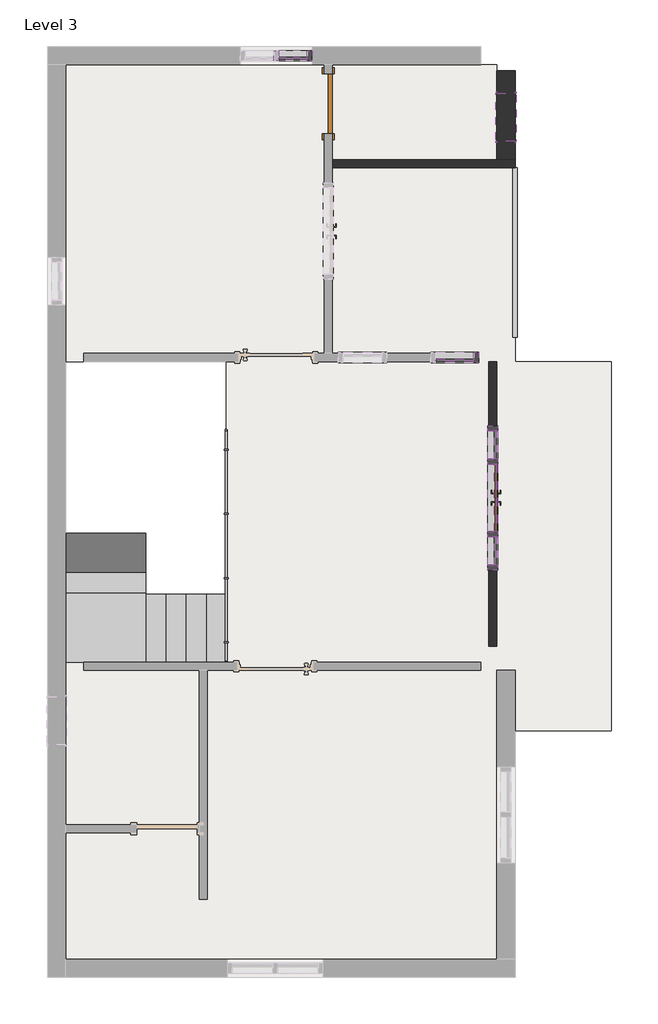
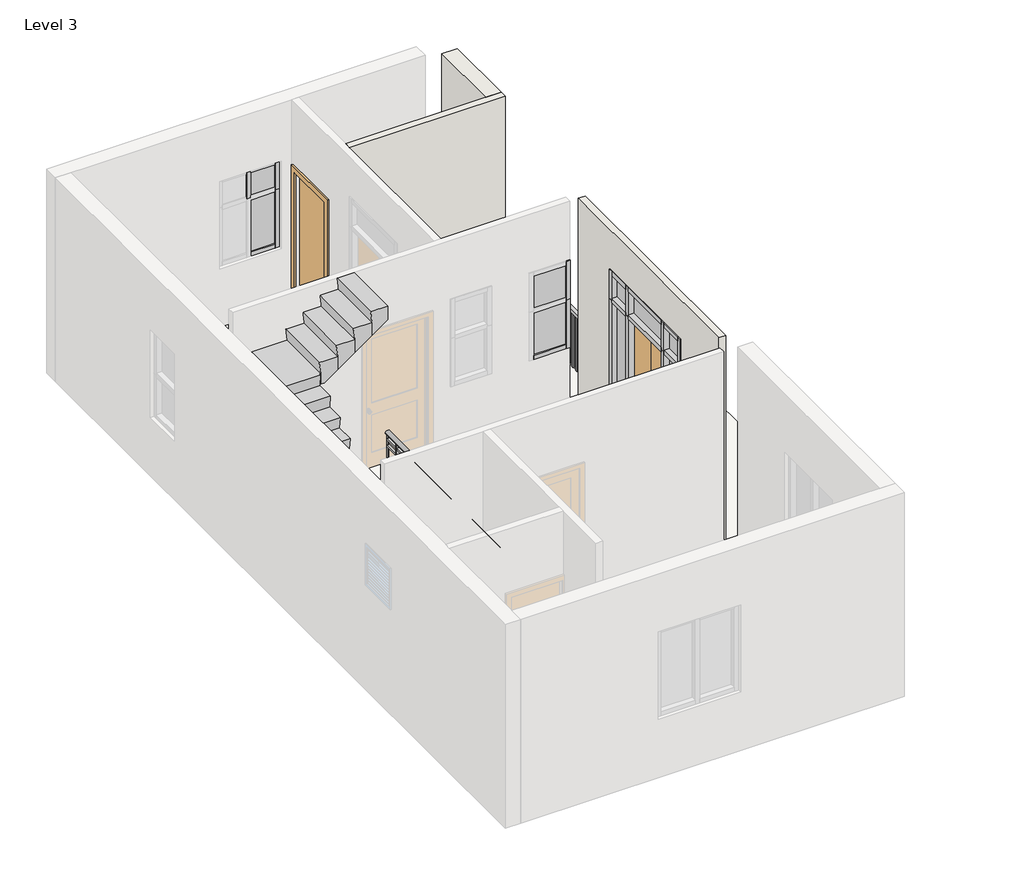
# One storey, part 2 of 2: 24 members, 9 plates, 3 walls, 2 doors, 2 railings, 1 slab, 1 stair flight, 1 window.
"""IFC4 building model written with IfcOpenShell, lengths in millimetres."""

from ifc_helpers import new_model, si_unit, point, frame, origin, place, context, project, spatial, polyline, ellipse_curve, trimmed, outline, extrude, faceted_brep, transform, mapped, element, save
from ifc_brep_helpers import plane_surface, extruded_surface, advanced_brep
from components import door_curtain_wall_double_glass_door_curtain_wall_double_88735db7, door_aa9e95e7, member_ffd4c858, member_15823cb3, member_843225dc, member_7cbddb58, member_af2f84b9, member_7db1855a, member_d2e7e466, member_3374d9b6, member_86d06fe4, member_47bfaf8a, member_aa870034, member_73c23c35, system_panel_glazed_a2bc0953, system_panel_glazed_235599b7, system_panel_glazed_0c1cb5df, system_panel_glazed_afbb4b88, system_panel_glazed_c43f0a09, system_panel_glazed_cc98a0ec, window_f2d8fef0

model = new_model("IFC4")

# Units and contexts
model_context = context("Model", 3, world=origin())
ifc_project = project(units=[si_unit("LENGTHUNIT", "METRE", prefix="MILLI")], contexts=[model_context])

# Site, building, storey
site = spatial("IfcSite", under=ifc_project)
building = spatial("IfcBuilding", under=site)
storey = spatial("IfcBuildingStorey", under=building, Name="Level 3", Elevation=3810.0)

# Doors
placement = place(None, origin())
door_curtain_wall_double_glass_door_curtain_wall_double_shape = door_curtain_wall_double_glass_door_curtain_wall_double_88735db7(model_context)
element("IfcDoor", 1, ObjectType="Door-Curtain-Wall-Double-Glass : Door-Curtain-Wall-Double-Glass", at=placement, inside=storey, context=model_context, shape_type="MappedRepresentation", body=[
    mapped(door_curtain_wall_double_glass_door_curtain_wall_double_shape, transform((576.4834347, 1882.9857557, 3873.5), x_axis=(0.0, -1.0, 0.0), y_axis=(1.0, 0.0, 0.0), z_axis=(0.0, 0.0, 1.0))),
])
door_shape = door_aa9e95e7(model_context)
element("IfcDoor", 2, ObjectType="Single-Flush : 2'6\" x7'", at=placement, inside=storey, context=model_context, shape_type="MappedRepresentation", body=[
    mapped(door_shape, transform((-1506.3165653, 6874.0857557, 3810.0), x_axis=(0.0, 1.0, 0.0), y_axis=(-1.0, 0.0, 0.0), z_axis=(0.0, 0.0, 1.0))),
])

# Members
member_shape = member_ffd4c858(model_context)
element("IfcMember", 3, ObjectType="Rectangular Mullion : 2.5\" x 5\" rectangular", at=placement, inside=storey, context=model_context, shape_type="MappedRepresentation", body=[
    mapped(member_shape, transform((576.4834347, 1425.7857557, 5943.6), x_axis=(0.0, -1.0, 0.0), y_axis=(-1.0, 0.0, 0.0), z_axis=(0.0, 0.0, -1.0))),
])
element("IfcMember", 4, ObjectType="Rectangular Mullion : 2.5\" x 5\" rectangular", at=placement, inside=storey, context=model_context, shape_type="MappedRepresentation", body=[
    mapped(member_shape, transform((576.4834347, 2340.1857557, 5943.6), x_axis=(0.0, -1.0, 0.0), y_axis=(-1.0, 0.0, 0.0), z_axis=(0.0, 0.0, -1.0))),
])
element("IfcMember", 5, ObjectType="Rectangular Mullion : 2.5\" x 5\" rectangular", at=placement, inside=storey, context=model_context, shape_type="MappedRepresentation", body=[
    mapped(member_shape, transform((-2166.7165653, 7483.6857557, 5638.8), x_axis=(-1.0, 0.0, 0.0), y_axis=(0.0, 1.0, 0.0), z_axis=(0.0, 0.0, -1.0))),
])
member_2_shape = member_15823cb3(model_context)
element("IfcMember", 6, ObjectType="Rectangular Mullion : 2.5\" x 5\" rectangular", at=placement, inside=storey, context=model_context, shape_type="MappedRepresentation", body=[
    mapped(member_2_shape, transform((576.4834347, 2797.3857557, 6400.8), x_axis=(0.0, 1.0, 0.0), y_axis=(-1.0, 0.0, 0.0), z_axis=(0.0, 0.0, 1.0))),
])
element("IfcMember", 7, ObjectType="Rectangular Mullion : 2.5\" x 5\" rectangular", at=placement, inside=storey, context=model_context, shape_type="MappedRepresentation", body=[
    mapped(member_2_shape, transform((-1709.5165653, 7483.6857557, 6096.0), x_axis=(1.0, 0.0, 0.0), y_axis=(0.0, 1.0, 0.0), z_axis=(0.0, 0.0, 1.0))),
])
element("IfcMember", 8, ObjectType="Rectangular Mullion : 2.5\" x 5\" rectangular", at=placement, inside=storey, context=model_context, shape_type="MappedRepresentation", body=[
    mapped(member_2_shape, transform((576.4834347, 968.5857557, 5943.6), x_axis=(0.0, -1.0, 0.0), y_axis=(-1.0, 0.0, 0.0), z_axis=(0.0, 0.0, -1.0))),
])
member_3_shape = member_843225dc(model_context)
element("IfcMember", 9, ObjectType="Rectangular Mullion : 2.5\" x 5\" rectangular", at=placement, inside=storey, context=model_context, shape_type="MappedRepresentation", body=[
    mapped(member_3_shape, transform((576.4834347, 1032.0857557, 6400.8), x_axis=(0.0, 0.0, 1.0), y_axis=(-1.0, 0.0, 0.0), z_axis=(0.0, -1.0, 0.0))),
])
element("IfcMember", 10, ObjectType="Rectangular Mullion : 2.5\" x 5\" rectangular", at=placement, inside=storey, context=model_context, shape_type="MappedRepresentation", body=[
    mapped(member_3_shape, transform((576.4834347, 2371.9357557, 6400.8), x_axis=(0.0, 0.0, 1.0), y_axis=(-1.0, 0.0, 0.0), z_axis=(0.0, -1.0, 0.0))),
])
element("IfcMember", 11, ObjectType="Rectangular Mullion : 2.5\" x 5\" rectangular", at=placement, inside=storey, context=model_context, shape_type="MappedRepresentation", body=[
    mapped(member_3_shape, transform((576.4834347, 2733.8857557, 3810.0), x_axis=(0.0, 0.0, -1.0), y_axis=(-1.0, 0.0, 0.0), z_axis=(0.0, 1.0, 0.0))),
])
element("IfcMember", 12, ObjectType="Rectangular Mullion : 2.5\" x 5\" rectangular", at=placement, inside=storey, context=model_context, shape_type="MappedRepresentation", body=[
    mapped(member_3_shape, transform((576.4834347, 1394.0357557, 3810.0), x_axis=(0.0, 0.0, -1.0), y_axis=(-1.0, 0.0, 0.0), z_axis=(0.0, 1.0, 0.0))),
])
element("IfcMember", 13, ObjectType="Rectangular Mullion : 2.5\" x 5\" rectangular", at=placement, inside=storey, context=model_context, shape_type="MappedRepresentation", body=[
    mapped(member_3_shape, transform((-1773.0165653, 7483.6857557, 4724.4), x_axis=(0.0, 0.0, -1.0), y_axis=(0.0, 1.0, 0.0), z_axis=(1.0, 0.0, 0.0))),
])
member_4_shape = member_7cbddb58(model_context)
element("IfcMember", 14, ObjectType="Rectangular Mullion : 2.5\" x 5\" rectangular", at=placement, inside=storey, context=model_context, shape_type="MappedRepresentation", body=[
    mapped(member_4_shape, transform((576.4834347, 1425.7857557, 3810.0), x_axis=(0.0, -1.0, 0.0), y_axis=(-1.0, 0.0, 0.0), z_axis=(0.0, 0.0, -1.0))),
])
element("IfcMember", 15, ObjectType="Rectangular Mullion : 2.5\" x 5\" rectangular", at=placement, inside=storey, context=model_context, shape_type="MappedRepresentation", body=[
    mapped(member_4_shape, transform((576.4834347, 2340.1857557, 3810.0), x_axis=(0.0, -1.0, 0.0), y_axis=(-1.0, 0.0, 0.0), z_axis=(0.0, 0.0, -1.0))),
])
member_5_shape = member_af2f84b9(model_context)
element("IfcMember", 16, ObjectType="Rectangular Mullion : 2.5\" x 5\" rectangular", at=placement, inside=storey, context=model_context, shape_type="MappedRepresentation", body=[
    mapped(member_5_shape, transform((576.4834347, 2371.9357557, 5943.6), x_axis=(0.0, 0.0, 1.0), y_axis=(-1.0, 0.0, 0.0), z_axis=(0.0, -1.0, 0.0))),
])
element("IfcMember", 17, ObjectType="Rectangular Mullion : 2.5\" x 5\" rectangular", at=placement, inside=storey, context=model_context, shape_type="MappedRepresentation", body=[
    mapped(member_5_shape, transform((576.4834347, 1032.0857557, 5943.6), x_axis=(0.0, 0.0, 1.0), y_axis=(-1.0, 0.0, 0.0), z_axis=(0.0, -1.0, 0.0))),
])
member_6_shape = member_7db1855a(model_context)
element("IfcMember", 18, ObjectType="Rectangular Mullion : 2.5\" x 5\" rectangular", at=placement, inside=storey, context=model_context, shape_type="MappedRepresentation", body=[
    mapped(member_6_shape, transform((576.4834347, 1457.5357557, 5943.6), x_axis=(0.0, 0.0, 1.0), y_axis=(-1.0, 0.0, 0.0), z_axis=(0.0, -1.0, 0.0))),
])
member_7_shape = member_d2e7e466(model_context)
element("IfcMember", 19, ObjectType="Rectangular Mullion : 2.5\" x 5\" rectangular", at=placement, inside=storey, context=model_context, shape_type="MappedRepresentation", body=[
    mapped(member_7_shape, transform((576.4834347, 2308.4357557, 3810.0), x_axis=(0.0, 0.0, -1.0), y_axis=(-1.0, 0.0, 0.0), z_axis=(0.0, 1.0, 0.0))),
])
element("IfcMember", 20, ObjectType="Rectangular Mullion : 2.5\" x 5\" rectangular", at=placement, inside=storey, context=model_context, shape_type="MappedRepresentation", body=[
    mapped(member_7_shape, transform((576.4834347, 1457.5357557, 6400.8), x_axis=(0.0, 0.0, 1.0), y_axis=(-1.0, 0.0, 0.0), z_axis=(0.0, -1.0, 0.0))),
])
member_8_shape = member_3374d9b6(model_context)
element("IfcMember", 21, ObjectType="Rectangular Mullion : 2.5\" x 5\" rectangular", at=placement, inside=storey, context=model_context, shape_type="MappedRepresentation", body=[
    mapped(member_8_shape, transform((576.4834347, 968.5857557, 3810.0), x_axis=(0.0, -1.0, 0.0), y_axis=(-1.0, 0.0, 0.0), z_axis=(0.0, 0.0, -1.0))),
])
element("IfcMember", 22, ObjectType="Rectangular Mullion : 2.5\" x 5\" rectangular", at=placement, inside=storey, context=model_context, shape_type="MappedRepresentation", body=[
    mapped(member_8_shape, transform((576.4834347, 2797.3857557, 5943.6), x_axis=(0.0, 1.0, 0.0), y_axis=(-1.0, 0.0, 0.0), z_axis=(0.0, 0.0, 1.0))),
])
member_9_shape = member_86d06fe4(model_context)
element("IfcMember", 23, ObjectType="Rectangular Mullion : 2.5\" x 5\" rectangular", at=placement, inside=storey, context=model_context, shape_type="MappedRepresentation", body=[
    mapped(member_9_shape, transform((335.1834347, 3660.9857557, 4724.4), x_axis=(0.0, 0.0, -1.0), y_axis=(0.0, 1.0, 0.0), z_axis=(1.0, 0.0, 0.0))),
])
member_10_shape = member_47bfaf8a(model_context)
element("IfcMember", 24, ObjectType="Rectangular Mullion : 2.5\" x 5\" rectangular", at=placement, inside=storey, context=model_context, shape_type="MappedRepresentation", body=[
    mapped(member_10_shape, transform((398.6834347, 3660.9857557, 6096.0), x_axis=(1.0, 0.0, 0.0), y_axis=(0.0, 1.0, 0.0), z_axis=(0.0, 0.0, 1.0))),
])
member_11_shape = member_aa870034(model_context)
element("IfcMember", 25, ObjectType="Rectangular Mullion : 2.5\" x 5\" rectangular", at=placement, inside=storey, context=model_context, shape_type="MappedRepresentation", body=[
    mapped(member_11_shape, transform((398.6834347, 3660.9857557, 5486.4), x_axis=(1.0, 0.0, 0.0), y_axis=(0.0, 1.0, 0.0), z_axis=(0.0, 0.0, 1.0))),
])
member_12_shape = member_73c23c35(model_context)
element("IfcMember", 26, ObjectType="Rectangular Mullion : 2.5\" x 5\" rectangular", at=placement, inside=storey, context=model_context, shape_type="MappedRepresentation", body=[
    mapped(member_12_shape, transform((-1709.5165653, 7483.6857557, 5638.8), x_axis=(1.0, 0.0, 0.0), y_axis=(0.0, 1.0, 0.0), z_axis=(0.0, 0.0, 1.0))),
])

# Plates
system_panel_glazed_shape = system_panel_glazed_a2bc0953(model_context)
element("IfcPlate", 27, ObjectType="System Panel : Glazed", at=placement, inside=storey, context=model_context, shape_type="MappedRepresentation", body=[
    mapped(system_panel_glazed_shape, transform((576.4834347, 2552.9107557, 3873.5), x_axis=(0.0, -1.0, 0.0), y_axis=(1.0, 0.0, 0.0), z_axis=(0.0, 0.0, 1.0))),
])
element("IfcPlate", 28, ObjectType="System Panel : Glazed", at=placement, inside=storey, context=model_context, shape_type="MappedRepresentation", body=[
    mapped(system_panel_glazed_shape, transform((576.4834347, 1213.0607557, 3873.5), x_axis=(0.0, -1.0, 0.0), y_axis=(1.0, 0.0, 0.0), z_axis=(0.0, 0.0, 1.0))),
])
system_panel_glazed_2_shape = system_panel_glazed_235599b7(model_context)
element("IfcPlate", 29, ObjectType="System Panel : Glazed", at=placement, inside=storey, context=model_context, shape_type="MappedRepresentation", body=[
    mapped(system_panel_glazed_2_shape, transform((576.4834347, 2552.9107557, 5975.35), x_axis=(0.0, -1.0, 0.0), y_axis=(1.0, 0.0, 0.0), z_axis=(0.0, 0.0, 1.0))),
])
element("IfcPlate", 30, ObjectType="System Panel : Glazed", at=placement, inside=storey, context=model_context, shape_type="MappedRepresentation", body=[
    mapped(system_panel_glazed_2_shape, transform((576.4834347, 1213.0607557, 5975.35), x_axis=(0.0, -1.0, 0.0), y_axis=(1.0, 0.0, 0.0), z_axis=(0.0, 0.0, 1.0))),
])
element("IfcPlate", 31, ObjectType="System Panel : Glazed", at=placement, inside=storey, context=model_context, shape_type="MappedRepresentation", body=[
    mapped(system_panel_glazed_2_shape, transform((-1953.9915653, 7483.6857557, 5670.55), x_axis=(-1.0, 0.0, 0.0), y_axis=(0.0, -1.0, 0.0), z_axis=(0.0, 0.0, 1.0))),
])
system_panel_glazed_3_shape = system_panel_glazed_0c1cb5df(model_context)
element("IfcPlate", 32, ObjectType="System Panel : Glazed", at=placement, inside=storey, context=model_context, shape_type="MappedRepresentation", body=[
    mapped(system_panel_glazed_3_shape, transform((576.4834347, 1882.9857557, 5975.35), x_axis=(0.0, -1.0, 0.0), y_axis=(1.0, 0.0, 0.0), z_axis=(0.0, 0.0, 1.0))),
])
system_panel_glazed_4_shape = system_panel_glazed_afbb4b88(model_context)
element("IfcPlate", 33, ObjectType="System Panel : Glazed", at=placement, inside=storey, context=model_context, shape_type="MappedRepresentation", body=[
    mapped(system_panel_glazed_4_shape, transform((93.8834347, 3660.9857557, 4787.9), x_axis=(-1.0, 0.0, 0.0), y_axis=(0.0, -1.0, 0.0), z_axis=(0.0, 0.0, 1.0))),
])
system_panel_glazed_5_shape = system_panel_glazed_c43f0a09(model_context)
element("IfcPlate", 34, ObjectType="System Panel : Glazed", at=placement, inside=storey, context=model_context, shape_type="MappedRepresentation", body=[
    mapped(system_panel_glazed_5_shape, transform((93.8834347, 3660.9857557, 5518.15), x_axis=(-1.0, 0.0, 0.0), y_axis=(0.0, -1.0, 0.0), z_axis=(0.0, 0.0, 1.0))),
])
system_panel_glazed_6_shape = system_panel_glazed_cc98a0ec(model_context)
element("IfcPlate", 35, ObjectType="System Panel : Glazed", at=placement, inside=storey, context=model_context, shape_type="MappedRepresentation", body=[
    mapped(system_panel_glazed_6_shape, transform((-1953.9915653, 7483.6857557, 4787.9), x_axis=(-1.0, 0.0, 0.0), y_axis=(0.0, -1.0, 0.0), z_axis=(0.0, 0.0, 1.0))),
])

# Railings
element("IfcRailing", 36, ObjectType="Glass Panel - Bottom Fill", at=placement, inside=storey, context=model_context, shape_type="SolidModel", body=[
    advanced_brep(
    [(-2763.6165653, 2746.5857557, 5029.2), (-2839.8165653, 2746.5857557, 5029.2), (-2763.6165653, -199.8142443, 5029.2), (-2839.8165653, -199.8142443, 5029.2)],
    [
        (0, 1, ellipse_curve(frame((-2801.7165653, 2746.5857557, 5029.2), z_axis=(0.0, 1.0, 0.0), x_axis=(-1.0, 0.0, 0.0)), 38.1, 28.575)),
        (1, 0, ellipse_curve(frame((-2801.7165653, 2746.5857557, 5029.2), z_axis=(0.0, 1.0, 0.0), x_axis=(-1.0, 0.0, 0.0)), 38.1, 28.575)),
        (2, 3, ellipse_curve(frame((-2801.7165653, -199.8142443, 5029.2), z_axis=(0.0, -1.0, 0.0), x_axis=(-1.0, 0.0, 0.0)), 38.1, 28.575)),
        (3, 2, ellipse_curve(frame((-2801.7165653, -199.8142443, 5029.2), z_axis=(0.0, -1.0, 0.0), x_axis=(-1.0, 0.0, 0.0)), 38.1, 28.575)),
        (0, 2),
        (3, 1),
    ],
    [
        plane_surface(frame((-2801.7165653, 2746.5857557, 5029.2), z_axis=(0.0, 1.0, 0.0), x_axis=(0.0, 0.0, -1.0))),
        plane_surface(frame((-2801.7165653, -199.8142443, 5029.2), z_axis=(0.0, -1.0, 0.0), x_axis=(0.0, 0.0, -1.0))),
        extruded_surface(trimmed(ellipse_curve(frame((-2801.7165653, -199.8142443, 5029.2), z_axis=(0.0, 1.0, 0.0), x_axis=(-1.0, 0.0, 0.0)), 38.1, 28.575), [point((-2763.6165653, -199.8142443, 5029.2))], [point((-2839.8165653, -199.8142443, 5029.2))], True, "CARTESIAN"), (0.0, 2946.4, 0.0), 2946.4),
        extruded_surface(trimmed(ellipse_curve(frame((-2801.7165653, -199.8142443, 5029.2), z_axis=(0.0, 1.0, 0.0), x_axis=(-1.0, 0.0, 0.0)), 38.1, 28.575), [point((-2839.8165653, -199.8142443, 5029.2))], [point((-2763.6165653, -199.8142443, 5029.2))], True, "CARTESIAN"), (0.0, 2946.4, 0.0), 2946.4),
    ],
    [
        (0, [[1, 2]]),
        (1, [[3, 4]]),
        (2, [[-1, 5, -4, 6]]),
        (3, [[-2, -6, -3, -5]]),
    ],
),
    extrude(outline(polyline([(-2814.4165653, 2746.5857557), (-2789.0165653, 2746.5857557), (-2789.0165653, -199.8142443), (-2814.4165653, -199.8142443), (-2814.4165653, 2746.5857557)])), frame((0.0, 0.0, 4914.9), z_axis=(0.0, 0.0, 1.0), x_axis=(1.0, 0.0, 0.0)), (0.0, 0.0, 1.0), 25.4),
    extrude(outline(polyline([(-2814.4165653, 2746.5857557), (-2789.0165653, 2746.5857557), (-2789.0165653, -199.8142443), (-2814.4165653, -199.8142443), (-2814.4165653, 2746.5857557)])), frame((0.0, 0.0, 4813.3), z_axis=(0.0, 0.0, 1.0), x_axis=(1.0, 0.0, 0.0)), (0.0, 0.0, 1.0), 25.4),
    extrude(outline(polyline([(-2827.1165653, 60.5357557), (-2776.3165653, 60.5357557), (-2776.3165653, 47.8357557), (-2827.1165653, 47.8357557), (-2827.1165653, 60.5357557)])), frame((0.0, 0.0, 4114.8), z_axis=(0.0, 0.0, 1.0), x_axis=(1.0, 0.0, 0.0)), (0.0, 0.0, 1.0), 885.825),
    extrude(outline(polyline([(-2795.1814083, 866.9857557), (-2795.1814083, 54.1857557), (-2801.5314083, 54.1857557), (-2801.5314083, 866.9857557), (-2795.1814083, 866.9857557)])), frame((0.0, 0.0, 4216.4), z_axis=(0.0, 0.0, 1.0), x_axis=(1.0, 0.0, 0.0)), (0.0, 0.0, 1.0), 596.9),
    extrude(outline(polyline([(-2827.1165653, 873.3357557), (-2776.3165653, 873.3357557), (-2776.3165653, 860.6357557), (-2827.1165653, 860.6357557), (-2827.1165653, 873.3357557)])), frame((0.0, 0.0, 4114.8), z_axis=(0.0, 0.0, 1.0), x_axis=(1.0, 0.0, 0.0)), (0.0, 0.0, 1.0), 885.825),
    extrude(outline(polyline([(-2795.1814083, 1679.7857557), (-2795.1814083, 866.9857557), (-2801.5314083, 866.9857557), (-2801.5314083, 1679.7857557), (-2795.1814083, 1679.7857557)])), frame((0.0, 0.0, 4216.4), z_axis=(0.0, 0.0, 1.0), x_axis=(1.0, 0.0, 0.0)), (0.0, 0.0, 1.0), 596.9),
    extrude(outline(polyline([(-2827.1165653, 1686.1357557), (-2776.3165653, 1686.1357557), (-2776.3165653, 1673.4357557), (-2827.1165653, 1673.4357557), (-2827.1165653, 1686.1357557)])), frame((0.0, 0.0, 4114.8), z_axis=(0.0, 0.0, 1.0), x_axis=(1.0, 0.0, 0.0)), (0.0, 0.0, 1.0), 885.825),
    extrude(outline(polyline([(-2795.1814083, 2492.5857557), (-2795.1814083, 1679.7857557), (-2801.5314083, 1679.7857557), (-2801.5314083, 2492.5857557), (-2795.1814083, 2492.5857557)])), frame((0.0, 0.0, 4216.4), z_axis=(0.0, 0.0, 1.0), x_axis=(1.0, 0.0, 0.0)), (0.0, 0.0, 1.0), 596.9),
    extrude(outline(polyline([(-2827.1165653, 2498.9357557), (-2776.3165653, 2498.9357557), (-2776.3165653, 2486.2357557), (-2827.1165653, 2486.2357557), (-2827.1165653, 2498.9357557)])), frame((0.0, 0.0, 4114.8), z_axis=(0.0, 0.0, 1.0), x_axis=(1.0, 0.0, 0.0)), (0.0, 0.0, 1.0), 885.825),
    extrude(outline(polyline([(-2811.2415653, -187.1142443), (-2792.1915653, -187.1142443), (-2792.1915653, -206.1642443), (-2811.2415653, -206.1642443), (-2811.2415653, -187.1142443)])), frame((0.0, 0.0, 4114.8), z_axis=(0.0, 0.0, 1.0), x_axis=(1.0, 0.0, 0.0)), (0.0, 0.0, 1.0), 885.825),
    extrude(outline(polyline([(-2811.2415653, 2752.9357557), (-2792.1915653, 2752.9357557), (-2792.1915653, 2733.8857557), (-2811.2415653, 2733.8857557), (-2811.2415653, 2752.9357557)])), frame((0.0, 0.0, 4114.8), z_axis=(0.0, 0.0, 1.0), x_axis=(1.0, 0.0, 0.0)), (0.0, 0.0, 1.0), 885.825),
])
element("IfcRailing", 37, ObjectType="Handrail - Rectangular", at=placement, inside=storey, context=model_context, shape_type="SweptSolid", body=[
    extrude(outline(polyline([(881.2834347, 3914.9857557), (830.4834347, 3914.9857557), (830.4834347, 6061.2857557), (881.2834347, 6061.2857557), (881.2834347, 3914.9857557)])), frame((0.0, 0.0, 4673.6), z_axis=(0.0, 0.0, 1.0), x_axis=(1.0, 0.0, 0.0)), (0.0, 0.0, 1.0), 50.8),
    extrude(outline(polyline([(865.4084347, 6039.0607557), (846.3584347, 6039.0607557), (846.3584347, 6058.1107557), (865.4084347, 6058.1107557), (865.4084347, 6039.0607557)])), frame((0.0, 0.0, 3810.0), z_axis=(0.0, 0.0, 1.0), x_axis=(1.0, 0.0, 0.0)), (0.0, 0.0, 1.0), 863.6),
    extrude(outline(polyline([(865.4084347, 5937.4607557), (846.3584347, 5937.4607557), (846.3584347, 5956.5107557), (865.4084347, 5956.5107557), (865.4084347, 5937.4607557)])), frame((0.0, 0.0, 3810.0), z_axis=(0.0, 0.0, 1.0), x_axis=(1.0, 0.0, 0.0)), (0.0, 0.0, 1.0), 863.6),
    extrude(outline(polyline([(865.4084347, 5835.8607557), (846.3584347, 5835.8607557), (846.3584347, 5854.9107557), (865.4084347, 5854.9107557), (865.4084347, 5835.8607557)])), frame((0.0, 0.0, 3810.0), z_axis=(0.0, 0.0, 1.0), x_axis=(1.0, 0.0, 0.0)), (0.0, 0.0, 1.0), 863.6),
    extrude(outline(polyline([(865.4084347, 5734.2607557), (846.3584347, 5734.2607557), (846.3584347, 5753.3107557), (865.4084347, 5753.3107557), (865.4084347, 5734.2607557)])), frame((0.0, 0.0, 3810.0), z_axis=(0.0, 0.0, 1.0), x_axis=(1.0, 0.0, 0.0)), (0.0, 0.0, 1.0), 863.6),
    extrude(outline(polyline([(865.4084347, 5632.6607557), (846.3584347, 5632.6607557), (846.3584347, 5651.7107557), (865.4084347, 5651.7107557), (865.4084347, 5632.6607557)])), frame((0.0, 0.0, 3810.0), z_axis=(0.0, 0.0, 1.0), x_axis=(1.0, 0.0, 0.0)), (0.0, 0.0, 1.0), 863.6),
    extrude(outline(polyline([(865.4084347, 5531.0607557), (846.3584347, 5531.0607557), (846.3584347, 5550.1107557), (865.4084347, 5550.1107557), (865.4084347, 5531.0607557)])), frame((0.0, 0.0, 3810.0), z_axis=(0.0, 0.0, 1.0), x_axis=(1.0, 0.0, 0.0)), (0.0, 0.0, 1.0), 863.6),
    extrude(outline(polyline([(865.4084347, 5429.4607557), (846.3584347, 5429.4607557), (846.3584347, 5448.5107557), (865.4084347, 5448.5107557), (865.4084347, 5429.4607557)])), frame((0.0, 0.0, 3810.0), z_axis=(0.0, 0.0, 1.0), x_axis=(1.0, 0.0, 0.0)), (0.0, 0.0, 1.0), 863.6),
    extrude(outline(polyline([(865.4084347, 5327.8607557), (846.3584347, 5327.8607557), (846.3584347, 5346.9107557), (865.4084347, 5346.9107557), (865.4084347, 5327.8607557)])), frame((0.0, 0.0, 3810.0), z_axis=(0.0, 0.0, 1.0), x_axis=(1.0, 0.0, 0.0)), (0.0, 0.0, 1.0), 863.6),
    extrude(outline(polyline([(865.4084347, 5226.2607557), (846.3584347, 5226.2607557), (846.3584347, 5245.3107557), (865.4084347, 5245.3107557), (865.4084347, 5226.2607557)])), frame((0.0, 0.0, 3810.0), z_axis=(0.0, 0.0, 1.0), x_axis=(1.0, 0.0, 0.0)), (0.0, 0.0, 1.0), 863.6),
    extrude(outline(polyline([(865.4084347, 5124.6607557), (846.3584347, 5124.6607557), (846.3584347, 5143.7107557), (865.4084347, 5143.7107557), (865.4084347, 5124.6607557)])), frame((0.0, 0.0, 3810.0), z_axis=(0.0, 0.0, 1.0), x_axis=(1.0, 0.0, 0.0)), (0.0, 0.0, 1.0), 863.6),
    extrude(outline(polyline([(865.4084347, 5023.0607557), (846.3584347, 5023.0607557), (846.3584347, 5042.1107557), (865.4084347, 5042.1107557), (865.4084347, 5023.0607557)])), frame((0.0, 0.0, 3810.0), z_axis=(0.0, 0.0, 1.0), x_axis=(1.0, 0.0, 0.0)), (0.0, 0.0, 1.0), 863.6),
    extrude(outline(polyline([(865.4084347, 4921.4607557), (846.3584347, 4921.4607557), (846.3584347, 4940.5107557), (865.4084347, 4940.5107557), (865.4084347, 4921.4607557)])), frame((0.0, 0.0, 3810.0), z_axis=(0.0, 0.0, 1.0), x_axis=(1.0, 0.0, 0.0)), (0.0, 0.0, 1.0), 863.6),
    extrude(outline(polyline([(865.4084347, 4819.8607557), (846.3584347, 4819.8607557), (846.3584347, 4838.9107557), (865.4084347, 4838.9107557), (865.4084347, 4819.8607557)])), frame((0.0, 0.0, 3810.0), z_axis=(0.0, 0.0, 1.0), x_axis=(1.0, 0.0, 0.0)), (0.0, 0.0, 1.0), 863.6),
    extrude(outline(polyline([(865.4084347, 4718.2607557), (846.3584347, 4718.2607557), (846.3584347, 4737.3107557), (865.4084347, 4737.3107557), (865.4084347, 4718.2607557)])), frame((0.0, 0.0, 3810.0), z_axis=(0.0, 0.0, 1.0), x_axis=(1.0, 0.0, 0.0)), (0.0, 0.0, 1.0), 863.6),
    extrude(outline(polyline([(865.4084347, 4616.6607557), (846.3584347, 4616.6607557), (846.3584347, 4635.7107557), (865.4084347, 4635.7107557), (865.4084347, 4616.6607557)])), frame((0.0, 0.0, 3810.0), z_axis=(0.0, 0.0, 1.0), x_axis=(1.0, 0.0, 0.0)), (0.0, 0.0, 1.0), 863.6),
    extrude(outline(polyline([(865.4084347, 4515.0607557), (846.3584347, 4515.0607557), (846.3584347, 4534.1107557), (865.4084347, 4534.1107557), (865.4084347, 4515.0607557)])), frame((0.0, 0.0, 3810.0), z_axis=(0.0, 0.0, 1.0), x_axis=(1.0, 0.0, 0.0)), (0.0, 0.0, 1.0), 863.6),
    extrude(outline(polyline([(865.4084347, 4413.4607557), (846.3584347, 4413.4607557), (846.3584347, 4432.5107557), (865.4084347, 4432.5107557), (865.4084347, 4413.4607557)])), frame((0.0, 0.0, 3810.0), z_axis=(0.0, 0.0, 1.0), x_axis=(1.0, 0.0, 0.0)), (0.0, 0.0, 1.0), 863.6),
    extrude(outline(polyline([(865.4084347, 4311.8607557), (846.3584347, 4311.8607557), (846.3584347, 4330.9107557), (865.4084347, 4330.9107557), (865.4084347, 4311.8607557)])), frame((0.0, 0.0, 3810.0), z_axis=(0.0, 0.0, 1.0), x_axis=(1.0, 0.0, 0.0)), (0.0, 0.0, 1.0), 863.6),
    extrude(outline(polyline([(865.4084347, 4210.2607557), (846.3584347, 4210.2607557), (846.3584347, 4229.3107557), (865.4084347, 4229.3107557), (865.4084347, 4210.2607557)])), frame((0.0, 0.0, 3810.0), z_axis=(0.0, 0.0, 1.0), x_axis=(1.0, 0.0, 0.0)), (0.0, 0.0, 1.0), 863.6),
    extrude(outline(polyline([(865.4084347, 4108.6607557), (846.3584347, 4108.6607557), (846.3584347, 4127.7107557), (865.4084347, 4127.7107557), (865.4084347, 4108.6607557)])), frame((0.0, 0.0, 3810.0), z_axis=(0.0, 0.0, 1.0), x_axis=(1.0, 0.0, 0.0)), (0.0, 0.0, 1.0), 863.6),
    extrude(outline(polyline([(865.4084347, 4007.0607557), (846.3584347, 4007.0607557), (846.3584347, 4026.1107557), (865.4084347, 4026.1107557), (865.4084347, 4007.0607557)])), frame((0.0, 0.0, 3810.0), z_axis=(0.0, 0.0, 1.0), x_axis=(1.0, 0.0, 0.0)), (0.0, 0.0, 1.0), 863.6),
    extrude(outline(polyline([(865.4084347, 6042.2357557), (846.3584347, 6042.2357557), (846.3584347, 6061.2857557), (865.4084347, 6061.2857557), (865.4084347, 6042.2357557)])), frame((0.0, 0.0, 3810.0), z_axis=(0.0, 0.0, 1.0), x_axis=(1.0, 0.0, 0.0)), (0.0, 0.0, 1.0), 863.6),
    extrude(outline(polyline([(865.4084347, 3914.9857557), (846.3584347, 3914.9857557), (846.3584347, 3934.0357557), (865.4084347, 3934.0357557), (865.4084347, 3914.9857557)])), frame((0.0, 0.0, 3810.0), z_axis=(0.0, 0.0, 1.0), x_axis=(1.0, 0.0, 0.0)), (0.0, 0.0, 1.0), 863.6),
])

# Slab
element("IfcSlab", 38, ObjectType="6\" floor", at=placement, inside=storey, context=model_context, shape_type="SweptSolid", body=[
    extrude(outline(polyline([(627.2834347, 7369.3857557), (627.2834347, 6061.2857557), (855.8834347, 6061.2857557), (855.8834347, 3610.1857557), (2075.0834347, 3610.1857557), (2075.0834347, -1063.4142443), (855.8834347, -1063.4142443), (855.8834347, -3959.0142443), (-4833.7165653, -3959.0142443), (-4833.7165653, -199.8142443), (-2801.7165653, -199.8142443), (-2801.7165653, 798.8688619), (-2801.7165653, 2893.0952618), (-2801.7165653, 3610.1857557), (-4833.7165653, 3610.1857557), (-4833.7165653, 7369.3857557), (627.2834347, 7369.3857557)])), frame((0.0, 0.0, 3657.6), z_axis=(0.0, 0.0, 1.0), x_axis=(1.0, 0.0, 0.0)), (0.0, 0.0, 1.0), 152.4),
])

# Stair flight
element("IfcStairFlight", 39, ObjectType="3/4\" Nosing 6 1/2\" Depth", at=placement, inside=storey, context=model_context, shape_type="Brep", body=[
    faceted_brep([(-2801.7165653, 663.7857557, 3987.8), (-2801.7165653, -199.8142443, 3987.8), (-2820.7665653, -199.8142443, 3810.0), (-2820.7665653, 663.7857557, 3810.0), (-3074.7665653, 663.7857557, 3987.8), (-3074.7665653, -199.8142443, 3987.8), (-3074.7665653, -199.8142443, 3810.0), (-3074.7665653, 663.7857557, 3810.0), (-3055.7165653, -199.8142443, 4165.6), (-3055.7165653, 663.7857557, 4165.6), (-3328.7665653, 663.7857557, 4165.6), (-3328.7665653, -199.8142443, 4165.6), (-3328.7665653, -199.8142443, 3964.0697668), (-3108.6668985, -199.8142443, 3810.0), (-3108.6668985, 663.7857557, 3810.0), (-3328.7665653, 663.7857557, 3964.0697668), (-3309.7165653, -199.8142443, 4343.4), (-3309.7165653, 663.7857557, 4343.4), (-3582.7665653, 663.7857557, 4343.4), (-3582.7665653, -199.8142443, 4343.4), (-3582.7665653, -199.8142443, 4141.8697668), (-3582.7665653, 663.7857557, 4141.8697668), (-3563.7165653, -199.8142443, 4521.2), (-3563.7165653, 663.7857557, 4521.2), (-3836.7665653, 663.7857557, 4521.2), (-3836.7665653, -199.8142443, 4521.2), (-3836.7665653, -199.8142443, 4319.6697668), (-4142.8097556, 663.7857557, 4533.9), (-3835.405851, 663.7857557, 4533.9), (-4833.7165653, 704.6678432, 4699.0), (-4833.7165653, -199.8142443, 4699.0), (-4142.8097556, -199.8142443, 4699.0), (-3817.7165653, -199.8142443, 4699.0), (-3817.7165653, 663.7857557, 4699.0), (-3817.7165653, 704.6678432, 4699.0), (-4833.7165653, 704.6678432, 4533.9), (-4833.7165653, -199.8142443, 4533.9), (-4142.8097556, -199.8142443, 4533.9), (-3817.7165653, 663.7857557, 4533.9), (-3817.7165653, 704.6678432, 4533.9), (-4833.7165653, 685.6178432, 4876.8), (-3817.7165653, 685.6178432, 4876.8), (-3817.7165653, 756.7110335, 4876.8), (-3817.7165653, 958.6678432, 4876.8), (-4833.7165653, 958.6678432, 4876.8), (-4833.7165653, 756.7110335, 4876.8), (-4833.7165653, 958.6678432, 4675.2697668), (-4833.7165653, 756.7110335, 4533.9), (-3817.7165653, 756.7110335, 4533.9), (-3817.7165653, 958.6678432, 4675.2697668), (-4833.7165653, 939.6178432, 5054.6), (-3817.7165653, 939.6178432, 5054.6), (-3817.7165653, 1212.6678432, 5054.6), (-4833.7165653, 1212.6678432, 5054.6), (-4833.7165653, 1212.6678432, 4853.0697668), (-3817.7165653, 1212.6678432, 4853.0697668), (-4833.7165653, 1193.6178432, 5232.4), (-3817.7165653, 1193.6178432, 5232.4), (-3817.7165653, 1466.6678432, 5232.4), (-4833.7165653, 1466.6678432, 5232.4), (-4833.7165653, 1466.6678432, 5030.8697668), (-3817.7165653, 1466.6678432, 5030.8697668), (-4833.7165653, 1447.6178432, 5410.2), (-3817.7165653, 1447.6178432, 5410.2), (-3817.7165653, 1720.6678432, 5410.2), (-4833.7165653, 1720.6678432, 5410.2), (-4833.7165653, 1720.6678432, 5208.6697668), (-3817.7165653, 1720.6678432, 5208.6697668), (-4833.7165653, 1701.6178432, 5588.0), (-3817.7165653, 1701.6178432, 5588.0), (-3817.7165653, 1974.6678432, 5588.0), (-4833.7165653, 1974.6678432, 5588.0), (-4833.7165653, 1974.6678432, 5386.4697668), (-3817.7165653, 1974.6678432, 5386.4697668), (-4833.7165653, 1955.6178432, 5765.8), (-3817.7165653, 1955.6178432, 5765.8), (-3817.7165653, 2228.6678432, 5765.8), (-4833.7165653, 2228.6678432, 5765.8), (-4833.7165653, 2228.6678432, 5564.2697668), (-3817.7165653, 2228.6678432, 5564.2697668), (-4833.7165653, 2209.6178432, 5943.6), (-3817.7165653, 2209.6178432, 5943.6), (-3817.7165653, 2482.6678432, 5943.6), (-4833.7165653, 2482.6678432, 5943.6), (-4833.7165653, 2482.6678432, 5742.0697668), (-3817.7165653, 2482.6678432, 5742.0697668), (-4833.7165653, 2463.6178432, 6121.4), (-3817.7165653, 2463.6178432, 6121.4), (-3817.7165653, 2736.6678432, 6121.4), (-4833.7165653, 2736.6678432, 6121.4), (-4833.7165653, 2736.6678432, 5919.8697668), (-3817.7165653, 2736.6678432, 5919.8697668), (-3798.6665653, 3610.1857557, 6299.2), (-4833.7165653, 3610.1857557, 6299.2), (-4833.7165653, 3042.7110335, 6299.2), (-4833.7165653, 2717.6178432, 6299.2), (-3817.7165653, 2717.6178432, 6299.2), (-3817.7165653, 2746.5857557, 6299.2), (-3798.6665653, 2746.5857557, 6299.2), (-3798.6665653, 3610.1857557, 6134.1), (-4833.7165653, 3610.1857557, 6134.1), (-4833.7165653, 3042.7110335, 6134.1), (-3817.7165653, 3042.7110335, 6134.1), (-3817.7165653, 2746.5857557, 6134.1), (-3798.6665653, 2746.5857557, 6134.1), (-3817.7165653, 3610.1857557, 6477.0), (-3817.7165653, 2746.5857557, 6477.0), (-3746.623375, 2746.5857557, 6477.0), (-3544.6665653, 2746.5857557, 6477.0), (-3544.6665653, 3610.1857557, 6477.0), (-3746.623375, 3610.1857557, 6477.0), (-3544.6665653, 3610.1857557, 6275.4697668), (-3746.623375, 3610.1857557, 6134.1), (-3746.623375, 2746.5857557, 6134.1), (-3544.6665653, 2746.5857557, 6275.4697668), (-3563.7165653, 3610.1857557, 6654.8), (-3563.7165653, 2746.5857557, 6654.8), (-3290.6665653, 2746.5857557, 6654.8), (-3290.6665653, 3610.1857557, 6654.8), (-3290.6665653, 3610.1857557, 6453.2697668), (-3290.6665653, 2746.5857557, 6453.2697668), (-3309.7165653, 3610.1857557, 6832.6), (-3309.7165653, 2746.5857557, 6832.6), (-3036.6665653, 2746.5857557, 6832.6), (-3036.6665653, 3610.1857557, 6832.6), (-3036.6665653, 3610.1857557, 6631.0697668), (-3036.6665653, 2746.5857557, 6631.0697668), (-3055.7165653, 3610.1857557, 7010.4), (-3055.7165653, 2746.5857557, 7010.4), (-2801.7165653, 2746.5857557, 7010.4), (-2801.7165653, 3610.1857557, 7010.4), (-2801.7165653, 3610.1857557, 6795.5347668), (-2801.7165653, 2746.5857557, 6795.5347668)], [[[0, 1, 2, 3]], [[1, 0, 4, 5]], [[1, 5, 6, 2]], [[4, 0, 3, 7]], [[8, 9, 10, 11]], [[6, 5, 8, 11, 12, 13]], [[4, 7, 14, 15, 10, 9]], [[5, 4, 9, 8]], [[16, 17, 18, 19]], [[16, 19, 20, 12, 11]], [[18, 17, 10, 15, 21]], [[11, 10, 17, 16]], [[22, 23, 24, 25]], [[22, 25, 26, 20, 19]], [[23, 18, 21, 27, 28, 24]], [[19, 18, 23, 22]], [[29, 30, 31, 32, 33, 34]], [[30, 29, 35, 36]], [[25, 32, 31, 30, 36, 37, 26]], [[33, 28, 38]], [[34, 33, 38, 39]], [[25, 24, 28, 33, 32]], [[40, 41, 42, 43, 44, 45]], [[29, 40, 45, 44, 46, 47, 35]], [[41, 34, 39, 48, 49, 43, 42]], [[29, 34, 41, 40]], [[50, 51, 52, 53]], [[50, 53, 54, 46, 44]], [[52, 51, 43, 49, 55]], [[44, 43, 51, 50]], [[56, 57, 58, 59]], [[56, 59, 60, 54, 53]], [[58, 57, 52, 55, 61]], [[53, 52, 57, 56]], [[62, 63, 64, 65]], [[62, 65, 66, 60, 59]], [[64, 63, 58, 61, 67]], [[59, 58, 63, 62]], [[68, 69, 70, 71]], [[68, 71, 72, 66, 65]], [[70, 69, 64, 67, 73]], [[65, 64, 69, 68]], [[74, 75, 76, 77]], [[74, 77, 78, 72, 71]], [[76, 75, 70, 73, 79]], [[71, 70, 75, 74]], [[80, 81, 82, 83]], [[80, 83, 84, 78, 77]], [[82, 81, 76, 79, 85]], [[77, 76, 81, 80]], [[86, 87, 88, 89]], [[86, 89, 90, 84, 83]], [[88, 87, 82, 85, 91]], [[83, 82, 87, 86]], [[92, 93, 94, 95, 96, 97, 98]], [[93, 92, 99, 100]], [[89, 95, 94, 93, 100, 101, 90]], [[97, 96, 88, 91, 102, 103]], [[98, 97, 103, 104]], [[89, 88, 96, 95]], [[105, 106, 107, 108, 109, 110]], [[92, 105, 110, 109, 111, 112, 99]], [[106, 98, 104, 113, 114, 108, 107]], [[92, 98, 106, 105]], [[115, 116, 117, 118]], [[115, 118, 119, 111, 109]], [[117, 116, 108, 114, 120]], [[109, 108, 116, 115]], [[121, 122, 123, 124]], [[121, 124, 125, 119, 118]], [[123, 122, 117, 120, 126]], [[118, 117, 122, 121]], [[127, 128, 129, 130]], [[127, 130, 131, 125, 124]], [[129, 128, 123, 126, 132]], [[130, 129, 132, 131]], [[124, 123, 128, 127]], [[2, 6, 13, 14, 7, 3]], [[37, 27, 21, 15, 14, 13, 12, 20, 26]], [[27, 37, 36, 35, 47, 48, 39, 38, 28]], [[48, 47, 46, 54, 60, 66, 72, 78, 84, 90, 101, 102, 91, 85, 79, 73, 67, 61, 55, 49]], [[102, 101, 100, 99, 112, 113, 104, 103]], [[113, 112, 111, 119, 125, 131, 132, 126, 120, 114]]]),
])

# Walls
element("IfcWall", 40, at=placement, inside=storey, context=model_context, shape_type="Brep", body=[
    faceted_brep([(-1455.5165653, 6061.2857557, 3810.0), (855.8834347, 6061.2857557, 3810.0), (855.8834347, 6061.2857557, 7010.4), (-1455.5165653, 6061.2857557, 7010.4), (-1455.5165653, 6162.8857557, 3810.0), (-1455.5165653, 6162.8857557, 7010.4), (627.2834347, 6162.8857557, 7010.4), (855.8834347, 6162.8857557, 7010.4), (855.8834347, 6162.8857557, 3810.0), (627.2834347, 6162.8857557, 3810.0)], [[[0, 1, 2, 3]], [[4, 5, 6, 7, 8, 9]], [[1, 0, 4, 9, 8]], [[3, 2, 7, 6, 5]], [[2, 1, 8, 7]], [[0, 3, 5, 4]]]),
])
element("IfcWall", 41, at=placement, inside=storey, context=model_context, shape_type="SweptSolid", body=[
    extrude(outline(polyline([(3.3857557, 3810.0), (3.3857557, 7010.4), (3610.1857557, 7010.4), (3610.1857557, 3810.0), (2797.3857557, 3810.0), (2797.3857557, 6400.8), (968.5857557, 6400.8), (968.5857557, 3810.0), (3.3857557, 3810.0)])), frame((525.6834347, 0.0, 0.0), z_axis=(1.0, 0.0, 0.0), x_axis=(0.0, 1.0, 0.0)), (0.0, 0.0, 1.0), 101.6),
])
element("IfcWall", 42, ObjectType="9\" wall", at=placement, inside=storey, context=model_context, shape_type="SweptSolid", body=[
    extrude(outline(polyline([(7293.1857557, 3810.0), (6162.8857557, 3810.0), (6162.8857557, 7010.4), (7293.1857557, 7010.4), (7293.1857557, 3810.0)]), holes=[polyline([(7007.4357557, 6096.0), (6397.8357557, 6096.0), (6397.8357557, 5486.4), (7007.4357557, 5486.4), (7007.4357557, 6096.0)])]), frame((627.2834347, 0.0, 0.0), z_axis=(1.0, 0.0, 0.0), x_axis=(0.0, 1.0, 0.0)), (0.0, 0.0, 1.0), 228.6),
])

# Window
window_shape = window_f2d8fef0(model_context)
element("IfcWindow", 43, ObjectType="Window-Louvers : 24\" x 24\"", at=placement, inside=storey, context=model_context, shape_type="MappedRepresentation", body=[
    mapped(window_shape, transform((747.9334347, 6702.6357557, 4572.0), x_axis=(0.0, -1.0, 0.0), y_axis=(1.0, 0.0, 0.0), z_axis=(0.0, 0.0, 1.0))),
])

save(model, "model.ifc")

# Revit data of these elements
# Type "Door-Curtain-Wall-Double-Glass : Door-Curtain-Wall-Double-Glass"
#   Type Mark = "16"
#   Assembly Code = "B2030100"
#   Analytic Construction = "<None>"
#   Width [instance default] = 6' - 0"
#   Thermal Resistance (R) = 10.0000 (h·ft²·°F)/BTU
#   Swing Angle [instance default] = 90.00°
#   Panel Width [instance default] = 3' - 0"
#   Offset = 0' - 2"
#   Heat Transfer Coefficient (U) = 0.1000 BTU/(h·ft²·°F)
#   Define Thermal Properties by = 1
#   Function = 1
#   Door Handle Material = Aluminum
#   Glazing = Glass
#   Visual Light Transmittance = 0
#   Solar Heat Gain Coefficient = 0
#   Construction Type Id = ""
# Type "Single-Flush : 2'6\" x7'"
#   Type Mark = "15"
#   Construction Type Id = "MDOOR"
#   Assembly Code = "C1020"
#   Analytic Construction = "Metal"
#   Thickness = 0' - 2"
#   Heat Transfer Coefficient (U) = 0.651978 BTU/(h·ft²·°F)
#   Height = 7' - 0"
#   Trim Projection Ext = 0' - 1"
#   Trim Projection Int = 0' - 1"
#   Trim Width = 0' - 3"
#   Width = 2' - 6"
#   Define Thermal Properties by = 1
#   Door Material = Door - Panel
#   Frame Material = Door - Frame
#   Visual Light Transmittance = 0
#   Solar Heat Gain Coefficient = 0
#   Function = (empty or 0)
#   Wall Closure = (empty or 0)
# Type "Rectangular Mullion : 2.5\" x 5\" rectangular"
#   built-in parameter 1007304 = 0.416667 (stored number, unit not read)
#   built-in parameter 1007301 = 0.104167 (stored number, unit not read)
#   built-in parameter 1007300 = 0.104167 (stored number, unit not read)
# Type "System Panel : Glazed"
#   Construction Type Id = "GSP4R"
#   Analytic Construction = "1/8 in Pilkington single glazing"
#   Visual Light Transmittance = 0.9
#   Solar Heat Gain Coefficient = 0.86
#   Heat Transfer Coefficient (U) = 1.18115 BTU/(h·ft²·°F)
#   Define Thermal Properties by = 1
# Type "Glass Panel - Bottom Fill"
#   Assembly Code = "C2010400"
#   built-in parameter 1008612 = 0.0416667 (stored number, unit not read)
#   built-in parameter 1008611 = 0.0416667 (stored number, unit not read)
#   built-in parameter 1008609 = 0.333333 (stored number, unit not read)
#   built-in parameter 1008604 = 0.166667 (stored number, unit not read)
#   built-in parameter 1008603 = 0.166667 (stored number, unit not read)
#   Railing Height = 3' - 0"
#   built-in parameter 1008630 = 2
#   built-in parameter 1008610 = 2
#   built-in parameter 1008618 = Baluster - Square : 3/4"
# Type "Handrail - Rectangular"
#   Assembly Code = "C2010400"
#   built-in parameter 1008612 = 0.0416667 (stored number, unit not read)
#   built-in parameter 1008611 = 0.0416667 (stored number, unit not read)
#   built-in parameter 1008609 = 0.333333 (stored number, unit not read)
#   built-in parameter 1008604 = 0.166667 (stored number, unit not read)
#   built-in parameter 1008603 = 0.166667 (stored number, unit not read)
#   Railing Height = 3' - 0"
#   built-in parameter 1008630 = 2
#   built-in parameter 1008610 = 2
#   built-in parameter 1008618 = Baluster - Square : 3/4"
# Type "6\" floor"
#   Assembly Code = "B1010"
#   Function = 0
#   Layers, outside or top first: 0' - 6" no material (function 1)
# Type
#   Assembly Code = "B2010"
#   Layers, outside or top first: 0' - 4" "01-9\" wall" (function 1)
# Type "9\" wall"
#   Assembly Code = "B2010"
#   Layers, outside or top first: 0' - 9" "01-9\" wall" (function 1)
# Type "Window-Louvers : 24\" x 24\""
#   Type Mark = "18"
#   Construction Type Id = "GSP4R"
#   Assembly Code = "B20"
#   Analytic Construction = "1/8 in Pilkington single glazing"
#   Visual Light Transmittance = 0.9
#   Thermal Resistance (R) = 1.53941 (h·ft²·°F)/BTU
#   Solar Heat Gain Coefficient = 0.78
#   Max Height = 1' - 11.74264"
#   Height = 2' - 0"
#   Heat Transfer Coefficient (U) = 0.6496 BTU/(h·ft²·°F)
#   Blade Width [instance default] = 1' - 10 1/2"
#   Blade Vertical Thickness = 0' - 0.35355"
#   Blade Thickness = 0' - 0 1/4"
#   Blade Spacing = 0' - 1 1/2"
#   Blade Height = 0' - 1.85355"
#   Blade Depth = 0' - 3"
#   Blade Angle = 45.00°
#   Default Sill Height = 3' - 0"
#   Trim Projection_Exterior = 0' - 0 1/2"
#   Trim Projection_Interior = 0' - 0 1/2"
#   Trim Width_Exterior = 0' - 1 1/2"
#   Trim Width_Interior = 0' - 1 1/2"
#   Width = 2' - 0"
#   Max Blade Count = 12
#   Define Thermal Properties by = 1
#   Blade Count = 12
#   Frame Material = Birch
#   Louver Material = Birch
#   Trim Exterior Material = Birch
#   Trim Interior Material = Birch
#   Wall Closure = (empty or 0)
# Element 1 (IfcDoor, "Door-Curtain-Wall-Double-Glass : Door-Curtain-Wall-Double-Glass")
#   Swing Angle = 90.00°
#   Phase Created = New Construction
#   Materials on its faces: "Aluminum", "Glass"
# Element 2 (IfcDoor, "Single-Flush : 2'6\" x7'")
#   Phase Created = New Construction
#   Materials on its faces: "Door - Frame", "Door - Panel"
# Elements 3, 4, 5, 6, 7, 8, 9, 10, 11, 12, 13, 14, 15, 16, 17, 18, 19, 20, 21, 22, 23, 24, 25, 26 (IfcMember, "Rectangular Mullion : 2.5\" x 5\" rectangular")
#   Phase Created = New Construction
#   Materials on its faces: "Aluminum"
# Elements 27, 28, 29, 30, 31, 32, 33, 34, 35 (IfcPlate, "System Panel : Glazed")
#   Phase Created = New Construction
#   Materials on its faces: "Glass"
# Element 36 (IfcRailing, "Glass Panel - Bottom Fill")
#   built-in parameter 1008621 = 1 (stored number, unit not read)
#   Phase Created = New Construction
#   Materials on its faces: "Glass"
# Element 37 (IfcRailing, "Handrail - Rectangular")
#   Phase Created = New Construction
# Element 38 (IfcSlab, "6\" floor")
#   Height Offset From Level = 0' - 0"
#   Phase Created = New Construction
#   Materials on its faces: "Default Floor"
# Element 39 (IfcStairFlight, "3/4\" Nosing 6 1/2\" Depth")
#   Phase Created = New Construction
#   Materials on its faces: "Concrete, Cast-in-Place gray"
# Elements 40, 41 (IfcWall)
#   Top Offset = 0' - 0"
#   Base Offset = 0' - 0"
#   wall height = 10' - 6"
#   Phase Created = New Construction
#   Base Constraint = Level 3
#   Top Constraint = Level 4
#   Materials on its faces: "01-9\" wall"
# Element 42 (IfcWall, "9\" wall")
#   Top Offset = 0' - 0"
#   Base Offset = 0' - 0"
#   wall height = 10' - 6"
#   Phase Created = New Construction
#   Base Constraint = Level 3
#   Top Constraint = Level 4
#   Materials on its faces: "01-9\" wall"
# Element 43 (IfcWindow, "Window-Louvers : 24\" x 24\"")
#   Mark = "2"
#   Blade Width = 1' - 10 1/2"
#   Phase Created = New Construction
#   Materials on its faces: "Birch"
# Materials
#   "Aluminum": class "Metal", colour RGB 247 247 247, transparency 0, Description = "Aluminum 6061", Cost = 0
#   "Glass": class "Glass", colour RGB 0 128 192, transparency 0.75, Description = "Soda Lime Glass", Cost = 0
#   "Door - Panel": class "Wood", colour RGB 210 159 95, transparency 0, Cost = 0
#   "Door - Frame": colour RGB 118 70 51, transparency 0, Cost = 0
#   "01-9\" wall": class "Generic", colour RGB 244 244 244, transparency 0, Cost = 0
#   "Birch": class "Wood", colour RGB 224 178 126, transparency 0, Description = "Betula Alleghaniensis", Cost = 0
#   "Default Floor": colour RGB 128 128 128, transparency 0, Cost = 0
#   "Concrete, Cast-in-Place gray": class "Concrete", colour RGB 192 192 192, transparency 0, Description = "Cast-in-place concrete", Cost = 0
